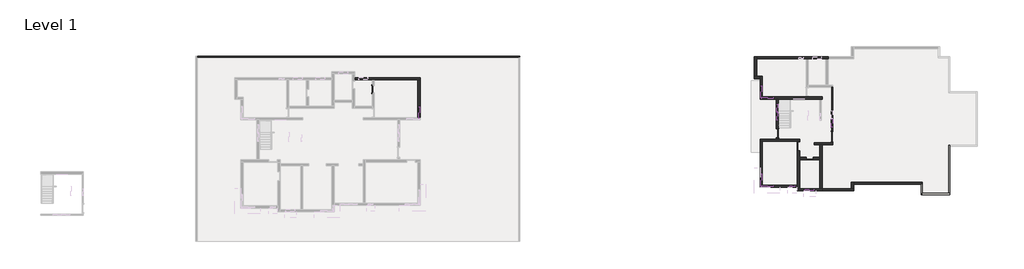
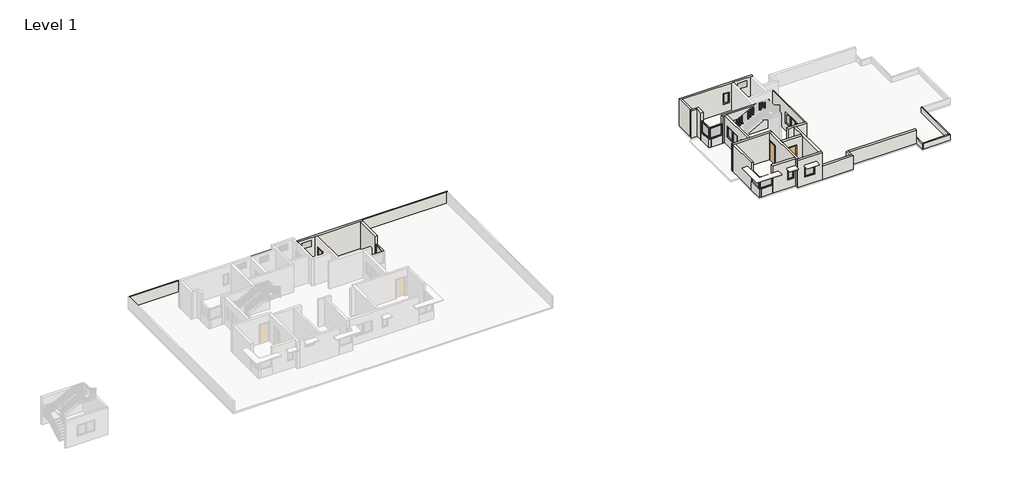
# One storey, part 3 of 9: 38 members, 29 walls, 12 plates, 5 doors.
"""IFC4 building model written with IfcOpenShell, lengths in millimetres."""

from ifc_helpers import new_model, si_unit, frame, origin, origin_with_axes, place, context, project, spatial, polyline, outline, extrude, faceted_brep, transform, mapped, element, save
from components import door_bb98abfd, single_flush_door_3_0ca8825f, door_e6ebe4aa, member_75074519, member_05917e3b, member_5783932f, member_49503176, member_cba00588, member_c17f1be2, member_2b49869a, member_8d24a278, member_86d06fe4, member_e557a406, system_panel_glazed_87944ff9, system_panel_glazed_c8a97ecb, system_panel_glazed_8ae75b46, system_panel_glazed_1b15d1ca, system_panel_glazed_cc4caca5, system_panel_glazed_25f99c47, system_panel_glazed_1bcf12e0, system_panel_glazed_610bb4e0

model = new_model("IFC4")

# Units and contexts
model_context = context("Model", 3, world=origin())
ifc_project = project(units=[si_unit("LENGTHUNIT", "METRE", prefix="MILLI")], contexts=[model_context])

# Site, building, storey
site = spatial("IfcSite", under=ifc_project)
building = spatial("IfcBuilding", under=site)
storey = spatial("IfcBuildingStorey", under=building, Name="Level 1", Elevation=0.0)

# Doors
placement = place(None, origin())
door_shape = door_bb98abfd(model_context)
element("IfcDoor", 1, ObjectType="Single-Flush : door 2'6\"", at=placement, inside=storey, context=model_context, shape_type="MappedRepresentation", body=[
    mapped(door_shape, transform((-29076.4146233, 18676.4624892, 0.0), x_axis=(0.0, 1.0, 0.0), y_axis=(-1.0, 0.0, 0.0), z_axis=(0.0, 0.0, 1.0))),
])
element("IfcDoor", 2, ObjectType="Single-Flush : door 2'6\"", at=placement, inside=storey, context=model_context, shape_type="MappedRepresentation", body=[
    mapped(door_shape, transform((16569.5100959, 11434.669664, 0.0), x_axis=(-1.0, 0.0, 0.0), y_axis=(0.0, -1.0, 0.0), z_axis=(0.0, 0.0, 1.0))),
])
single_flush_door_3_shape = single_flush_door_3_0ca8825f(model_context)
element("IfcDoor", 3, ObjectType="Single-Flush : door 3'", at=placement, inside=storey, context=model_context, shape_type="MappedRepresentation", body=[
    mapped(single_flush_door_3_shape, transform((13178.6100959, 14076.3480703, 0.0), x_axis=(0.0, -1.0, 0.0), y_axis=(1.0, 0.0, 0.0), z_axis=(0.0, 0.0, 1.0))),
])
element("IfcDoor", 4, ObjectType="Single-Flush : door 3'", at=placement, inside=storey, context=model_context, shape_type="MappedRepresentation", body=[
    mapped(single_flush_door_3_shape, transform((15388.4100959, 12704.7480703, 0.0), x_axis=(0.0, 1.0, 0.0), y_axis=(-1.0, 0.0, 0.0), z_axis=(0.0, 0.0, 1.0))),
])
door_2_shape = door_e6ebe4aa(model_context)
element("IfcDoor", 5, ObjectType="Single-Flush : door 3'6\"", at=placement, inside=storey, context=model_context, shape_type="MappedRepresentation", body=[
    mapped(door_2_shape, transform((18912.6600959, 13695.3480703, 0.0), x_axis=(0.0, -1.0, 0.0), y_axis=(1.0, 0.0, 0.0), z_axis=(0.0, 0.0, 1.0))),
])

# Members
member_shape = member_75074519(model_context)
element("IfcMember", 6, ObjectType="Rectangular Mullion : 2.5\" x 5\" rectangular", at=placement, inside=storey, context=model_context, shape_type="MappedRepresentation", body=[
    mapped(member_shape, transform((-24263.1146233, 16911.1624892, 914.4), x_axis=(0.0, 1.0, 0.0), y_axis=(1.0, 0.0, 0.0), z_axis=(0.0, 0.0, -1.0))),
])
element("IfcMember", 7, ObjectType="Rectangular Mullion : 2.5\" x 5\" rectangular", at=placement, inside=storey, context=model_context, shape_type="MappedRepresentation", body=[
    mapped(member_shape, transform((11486.0219681, 17689.4980703, 914.4), x_axis=(0.0, -1.0, 0.0), y_axis=(-1.0, 0.0, 0.0), z_axis=(0.0, 0.0, -1.0))),
])
element("IfcMember", 8, ObjectType="Rectangular Mullion : 2.5\" x 5\" rectangular", at=placement, inside=storey, context=model_context, shape_type="MappedRepresentation", body=[
    mapped(member_shape, transform((12835.7100959, 17752.9980703, 914.4), x_axis=(1.0, 0.0, 0.0), y_axis=(0.0, -1.0, 0.0), z_axis=(0.0, 0.0, -1.0))),
])
element("IfcMember", 9, ObjectType="Rectangular Mullion : 2.5\" x 5\" rectangular", at=placement, inside=storey, context=model_context, shape_type="MappedRepresentation", body=[
    mapped(member_shape, transform((11486.0219681, 8462.949831, 914.4), x_axis=(0.0, -1.0, 0.0), y_axis=(-1.0, 0.0, 0.0), z_axis=(0.0, 0.0, -1.0))),
])
element("IfcMember", 10, ObjectType="Rectangular Mullion : 2.5\" x 5\" rectangular", at=placement, inside=storey, context=model_context, shape_type="MappedRepresentation", body=[
    mapped(member_shape, transform((12835.7100959, 8526.449831, 914.4), x_axis=(1.0, 0.0, 0.0), y_axis=(0.0, -1.0, 0.0), z_axis=(0.0, 0.0, -1.0))),
])
element("IfcMember", 11, ObjectType="Rectangular Mullion : 2.5\" x 5\" rectangular", at=placement, inside=storey, context=model_context, shape_type="MappedRepresentation", body=[
    mapped(member_shape, transform((15045.5100959, 8513.7480703, 914.4), x_axis=(1.0, 0.0, 0.0), y_axis=(0.0, -1.0, 0.0), z_axis=(0.0, 0.0, -1.0))),
])
element("IfcMember", 12, ObjectType="Rectangular Mullion : 2.5\" x 5\" rectangular", at=placement, inside=storey, context=model_context, shape_type="MappedRepresentation", body=[
    mapped(member_shape, transform((17064.8100959, 8132.669664, 914.4), x_axis=(1.0, 0.0, 0.0), y_axis=(0.0, -1.0, 0.0), z_axis=(0.0, 0.0, -1.0))),
])
element("IfcMember", 13, ObjectType="Rectangular Mullion : 2.5\" x 5\" rectangular", at=placement, inside=storey, context=model_context, shape_type="MappedRepresentation", body=[
    mapped(member_shape, transform((11486.0219681, 19092.8480703, 2133.6), x_axis=(0.0, 1.0, 0.0), y_axis=(-1.0, 0.0, 0.0), z_axis=(0.0, 0.0, 1.0))),
])
element("IfcMember", 14, ObjectType="Rectangular Mullion : 2.5\" x 5\" rectangular", at=placement, inside=storey, context=model_context, shape_type="MappedRepresentation", body=[
    mapped(member_shape, transform((11486.0219681, 17752.9980703, 2133.6), x_axis=(-1.0, 0.0, 0.0), y_axis=(0.0, -1.0, 0.0), z_axis=(0.0, 0.0, 1.0))),
])
element("IfcMember", 15, ObjectType="Rectangular Mullion : 2.5\" x 5\" rectangular", at=placement, inside=storey, context=model_context, shape_type="MappedRepresentation", body=[
    mapped(member_shape, transform((11486.0219681, 9872.649831, 2133.6), x_axis=(0.0, 1.0, 0.0), y_axis=(-1.0, 0.0, 0.0), z_axis=(0.0, 0.0, 1.0))),
])
element("IfcMember", 16, ObjectType="Rectangular Mullion : 2.5\" x 5\" rectangular", at=placement, inside=storey, context=model_context, shape_type="MappedRepresentation", body=[
    mapped(member_shape, transform((11486.0219681, 8526.449831, 2133.6), x_axis=(-1.0, 0.0, 0.0), y_axis=(0.0, -1.0, 0.0), z_axis=(0.0, 0.0, 1.0))),
])
element("IfcMember", 17, ObjectType="Rectangular Mullion : 2.5\" x 5\" rectangular", at=placement, inside=storey, context=model_context, shape_type="MappedRepresentation", body=[
    mapped(member_shape, transform((14435.9100959, 8513.7480703, 2133.6), x_axis=(-1.0, 0.0, 0.0), y_axis=(0.0, -1.0, 0.0), z_axis=(0.0, 0.0, 1.0))),
])
element("IfcMember", 18, ObjectType="Rectangular Mullion : 2.5\" x 5\" rectangular", at=placement, inside=storey, context=model_context, shape_type="MappedRepresentation", body=[
    mapped(member_shape, transform((15998.0100959, 8132.669664, 2133.6), x_axis=(-1.0, 0.0, 0.0), y_axis=(0.0, -1.0, 0.0), z_axis=(0.0, 0.0, 1.0))),
])
member_2_shape = member_05917e3b(model_context)
element("IfcMember", 19, ObjectType="Rectangular Mullion : 2.5\" x 5\" rectangular", at=placement, inside=storey, context=model_context, shape_type="MappedRepresentation", body=[
    mapped(member_2_shape, transform((12772.2100959, 17752.9980703, 2133.6), x_axis=(0.0, 0.0, 1.0), y_axis=(0.0, -1.0, 0.0), z_axis=(1.0, 0.0, 0.0))),
])
element("IfcMember", 20, ObjectType="Rectangular Mullion : 2.5\" x 5\" rectangular", at=placement, inside=storey, context=model_context, shape_type="MappedRepresentation", body=[
    mapped(member_2_shape, transform((12772.2100959, 8526.449831, 2133.6), x_axis=(0.0, 0.0, 1.0), y_axis=(0.0, -1.0, 0.0), z_axis=(1.0, 0.0, 0.0))),
])
element("IfcMember", 21, ObjectType="Rectangular Mullion : 2.5\" x 5\" rectangular", at=placement, inside=storey, context=model_context, shape_type="MappedRepresentation", body=[
    mapped(member_2_shape, transform((11549.5219681, 17752.9980703, 914.4), x_axis=(0.0, 0.0, -1.0), y_axis=(0.0, -1.0, 0.0), z_axis=(-1.0, 0.0, 0.0))),
])
element("IfcMember", 22, ObjectType="Rectangular Mullion : 2.5\" x 5\" rectangular", at=placement, inside=storey, context=model_context, shape_type="MappedRepresentation", body=[
    mapped(member_2_shape, transform((11549.5219681, 8526.449831, 914.4), x_axis=(0.0, 0.0, -1.0), y_axis=(0.0, -1.0, 0.0), z_axis=(-1.0, 0.0, 0.0))),
])
member_3_shape = member_5783932f(model_context)
element("IfcMember", 23, ObjectType="Rectangular Mullion : 2.5\" x 5\" rectangular", at=placement, inside=storey, context=model_context, shape_type="MappedRepresentation", body=[
    mapped(member_3_shape, transform((11486.0219681, 8526.449831, 2133.6), x_axis=(0.0, 0.0, 1.0), y_axis=(-1.0, 0.0, 0.0), z_axis=(0.0, -1.0, 0.0))),
])
element("IfcMember", 24, ObjectType="Rectangular Mullion : 2.5\" x 5\" rectangular", at=placement, inside=storey, context=model_context, shape_type="MappedRepresentation", body=[
    mapped(member_3_shape, transform((11486.0219681, 9809.149831, 914.4), x_axis=(0.0, 0.0, -1.0), y_axis=(-1.0, 0.0, 0.0), z_axis=(0.0, 1.0, 0.0))),
])
member_4_shape = member_49503176(model_context)
element("IfcMember", 25, ObjectType="Rectangular Mullion : 2.5\" x 5\" rectangular", at=placement, inside=storey, context=model_context, shape_type="MappedRepresentation", body=[
    mapped(member_4_shape, transform((-24263.1146233, 16847.6624892, 2133.6), x_axis=(0.0, 0.0, 1.0), y_axis=(1.0, 0.0, 0.0), z_axis=(0.0, 1.0, 0.0))),
])
member_5_shape = member_cba00588(model_context)
element("IfcMember", 26, ObjectType="Rectangular Mullion : 2.5\" x 5\" rectangular", at=placement, inside=storey, context=model_context, shape_type="MappedRepresentation", body=[
    mapped(member_5_shape, transform((11486.0219681, 17752.9980703, 2133.6), x_axis=(0.0, 0.0, 1.0), y_axis=(-1.0, 0.0, 0.0), z_axis=(0.0, -1.0, 0.0))),
])
element("IfcMember", 27, ObjectType="Rectangular Mullion : 2.5\" x 5\" rectangular", at=placement, inside=storey, context=model_context, shape_type="MappedRepresentation", body=[
    mapped(member_5_shape, transform((11486.0219681, 19029.3480703, 914.4), x_axis=(0.0, 0.0, -1.0), y_axis=(-1.0, 0.0, 0.0), z_axis=(0.0, 1.0, 0.0))),
])
member_6_shape = member_c17f1be2(model_context)
element("IfcMember", 28, ObjectType="Rectangular Mullion : 2.5\" x 5\" rectangular", at=placement, inside=storey, context=model_context, shape_type="MappedRepresentation", body=[
    mapped(member_6_shape, transform((13162.4368388, 17124.3480703, 2133.6), x_axis=(0.0, 0.0, 1.0), y_axis=(1.0, 0.0, 0.0), z_axis=(0.0, 1.0, 0.0))),
])
element("IfcMember", 29, ObjectType="Rectangular Mullion : 2.5\" x 5\" rectangular", at=placement, inside=storey, context=model_context, shape_type="MappedRepresentation", body=[
    mapped(member_6_shape, transform((13162.4368388, 16241.6980703, 2133.6), x_axis=(0.0, 0.0, 1.0), y_axis=(1.0, 0.0, 0.0), z_axis=(0.0, 1.0, 0.0))),
])
element("IfcMember", 30, ObjectType="Rectangular Mullion : 2.5\" x 5\" rectangular", at=placement, inside=storey, context=model_context, shape_type="MappedRepresentation", body=[
    mapped(member_6_shape, transform((13162.4368388, 15422.5480703, 914.4), x_axis=(0.0, 0.0, -1.0), y_axis=(1.0, 0.0, 0.0), z_axis=(0.0, -1.0, 0.0))),
])
element("IfcMember", 31, ObjectType="Rectangular Mullion : 2.5\" x 5\" rectangular", at=placement, inside=storey, context=model_context, shape_type="MappedRepresentation", body=[
    mapped(member_6_shape, transform((13162.4368388, 16305.1980703, 914.4), x_axis=(0.0, 0.0, -1.0), y_axis=(1.0, 0.0, 0.0), z_axis=(0.0, -1.0, 0.0))),
])
member_7_shape = member_2b49869a(model_context)
element("IfcMember", 32, ObjectType="Rectangular Mullion : 2.5\" x 5\" rectangular", at=placement, inside=storey, context=model_context, shape_type="MappedRepresentation", body=[
    mapped(member_7_shape, transform((13162.4368388, 16273.4480703, 914.4), x_axis=(0.0, 1.0, 0.0), y_axis=(1.0, 0.0, 0.0), z_axis=(0.0, 0.0, -1.0))),
])
element("IfcMember", 33, ObjectType="Rectangular Mullion : 2.5\" x 5\" rectangular", at=placement, inside=storey, context=model_context, shape_type="MappedRepresentation", body=[
    mapped(member_7_shape, transform((18890.1839667, 15549.2510521, 914.4), x_axis=(0.0, 1.0, 0.0), y_axis=(1.0, 0.0, 0.0), z_axis=(0.0, 0.0, -1.0))),
])
element("IfcMember", 34, ObjectType="Rectangular Mullion : 2.5\" x 5\" rectangular", at=placement, inside=storey, context=model_context, shape_type="MappedRepresentation", body=[
    mapped(member_shape, transform((13162.4368388, 17187.8480703, 914.4), x_axis=(0.0, 1.0, 0.0), y_axis=(1.0, 0.0, 0.0), z_axis=(0.0, 0.0, -1.0))),
])
element("IfcMember", 35, ObjectType="Rectangular Mullion : 2.5\" x 5\" rectangular", at=placement, inside=storey, context=model_context, shape_type="MappedRepresentation", body=[
    mapped(member_shape, transform((13162.4368388, 15359.0480703, 2133.6), x_axis=(0.0, -1.0, 0.0), y_axis=(1.0, 0.0, 0.0), z_axis=(0.0, 0.0, 1.0))),
])
element("IfcMember", 36, ObjectType="Rectangular Mullion : 2.5\" x 5\" rectangular", at=placement, inside=storey, context=model_context, shape_type="MappedRepresentation", body=[
    mapped(member_shape, transform((18890.1839667, 14635.1480703, 2133.6), x_axis=(0.0, -1.0, 0.0), y_axis=(1.0, 0.0, 0.0), z_axis=(0.0, 0.0, 1.0))),
])
member_8_shape = member_8d24a278(model_context)
element("IfcMember", 37, ObjectType="Rectangular Mullion : 2.5\" x 5\" rectangular", at=placement, inside=storey, context=model_context, shape_type="MappedRepresentation", body=[
    mapped(member_8_shape, transform((18890.1839667, 15517.5010521, 2133.6), x_axis=(0.0, 0.0, 1.0), y_axis=(1.0, 0.0, 0.0), z_axis=(0.0, 1.0, 0.0))),
])
element("IfcMember", 38, ObjectType="Rectangular Mullion : 2.5\" x 5\" rectangular", at=placement, inside=storey, context=model_context, shape_type="MappedRepresentation", body=[
    mapped(member_8_shape, transform((18890.1839667, 14698.6480703, 914.4), x_axis=(0.0, 0.0, -1.0), y_axis=(1.0, 0.0, 0.0), z_axis=(0.0, -1.0, 0.0))),
])
element("IfcMember", 39, ObjectType="Rectangular Mullion : 2.5\" x 5\" rectangular", at=placement, inside=storey, context=model_context, shape_type="MappedRepresentation", body=[
    mapped(member_8_shape, transform((18890.1839667, 15581.0010521, 914.4), x_axis=(0.0, 0.0, -1.0), y_axis=(1.0, 0.0, 0.0), z_axis=(0.0, -1.0, 0.0))),
])
member_9_shape = member_86d06fe4(model_context)
element("IfcMember", 40, ObjectType="Rectangular Mullion : 2.5\" x 5\" rectangular", at=placement, inside=storey, context=model_context, shape_type="MappedRepresentation", body=[
    mapped(member_9_shape, transform((14982.0100959, 8513.7480703, 2133.6), x_axis=(0.0, 0.0, 1.0), y_axis=(0.0, -1.0, 0.0), z_axis=(1.0, 0.0, 0.0))),
])
element("IfcMember", 41, ObjectType="Rectangular Mullion : 2.5\" x 5\" rectangular", at=placement, inside=storey, context=model_context, shape_type="MappedRepresentation", body=[
    mapped(member_9_shape, transform((14499.4100959, 8513.7480703, 914.4), x_axis=(0.0, 0.0, -1.0), y_axis=(0.0, -1.0, 0.0), z_axis=(-1.0, 0.0, 0.0))),
])
member_10_shape = member_e557a406(model_context)
element("IfcMember", 42, ObjectType="Rectangular Mullion : 2.5\" x 5\" rectangular", at=placement, inside=storey, context=model_context, shape_type="MappedRepresentation", body=[
    mapped(member_10_shape, transform((17001.3100959, 8132.669664, 2133.6), x_axis=(0.0, 0.0, 1.0), y_axis=(0.0, -1.0, 0.0), z_axis=(1.0, 0.0, 0.0))),
])
element("IfcMember", 43, ObjectType="Rectangular Mullion : 2.5\" x 5\" rectangular", at=placement, inside=storey, context=model_context, shape_type="MappedRepresentation", body=[
    mapped(member_10_shape, transform((16061.5100959, 8132.669664, 914.4), x_axis=(0.0, 0.0, -1.0), y_axis=(0.0, -1.0, 0.0), z_axis=(-1.0, 0.0, 0.0))),
])

# Plates
system_panel_glazed_shape = system_panel_glazed_87944ff9(model_context)
element("IfcPlate", 44, ObjectType="System Panel : Glazed", at=placement, inside=storey, context=model_context, shape_type="MappedRepresentation", body=[
    mapped(system_panel_glazed_shape, transform((11486.0219681, 9167.799831, 977.9), x_axis=(0.0, -1.0, 0.0), y_axis=(1.0, 0.0, 0.0), z_axis=(0.0, 0.0, 1.0))),
])
system_panel_glazed_2_shape = system_panel_glazed_c8a97ecb(model_context)
element("IfcPlate", 45, ObjectType="System Panel : Glazed", at=placement, inside=storey, context=model_context, shape_type="MappedRepresentation", body=[
    mapped(system_panel_glazed_2_shape, transform((12160.866032, 17752.9980703, 977.9), x_axis=(1.0, 0.0, 0.0), y_axis=(0.0, 1.0, 0.0), z_axis=(0.0, 0.0, 1.0))),
])
element("IfcPlate", 46, ObjectType="System Panel : Glazed", at=placement, inside=storey, context=model_context, shape_type="MappedRepresentation", body=[
    mapped(system_panel_glazed_2_shape, transform((12160.866032, 8526.449831, 977.9), x_axis=(1.0, 0.0, 0.0), y_axis=(0.0, 1.0, 0.0), z_axis=(0.0, 0.0, 1.0))),
])
system_panel_glazed_3_shape = system_panel_glazed_8ae75b46(model_context)
element("IfcPlate", 47, ObjectType="System Panel : Glazed", at=placement, inside=storey, context=model_context, shape_type="MappedRepresentation", body=[
    mapped(system_panel_glazed_3_shape, transform((-24263.1146233, 16231.7124892, 977.9), x_axis=(0.0, 1.0, 0.0), y_axis=(-1.0, 0.0, 0.0), z_axis=(0.0, 0.0, 1.0))),
])
system_panel_glazed_4_shape = system_panel_glazed_1b15d1ca(model_context)
element("IfcPlate", 48, ObjectType="System Panel : Glazed", at=placement, inside=storey, context=model_context, shape_type="MappedRepresentation", body=[
    mapped(system_panel_glazed_4_shape, transform((11486.0219681, 18391.1730703, 977.9), x_axis=(0.0, -1.0, 0.0), y_axis=(1.0, 0.0, 0.0), z_axis=(0.0, 0.0, 1.0))),
])
system_panel_glazed_5_shape = system_panel_glazed_cc4caca5(model_context)
element("IfcPlate", 49, ObjectType="System Panel : Glazed", at=placement, inside=storey, context=model_context, shape_type="MappedRepresentation", body=[
    mapped(system_panel_glazed_5_shape, transform((13162.4368388, 15832.1230703, 977.9), x_axis=(0.0, 1.0, 0.0), y_axis=(-1.0, 0.0, 0.0), z_axis=(0.0, 0.0, 1.0))),
])
element("IfcPlate", 50, ObjectType="System Panel : Glazed", at=placement, inside=storey, context=model_context, shape_type="MappedRepresentation", body=[
    mapped(system_panel_glazed_5_shape, transform((13162.4368388, 16714.7730703, 977.9), x_axis=(0.0, 1.0, 0.0), y_axis=(-1.0, 0.0, 0.0), z_axis=(0.0, 0.0, 1.0))),
])
system_panel_glazed_6_shape = system_panel_glazed_25f99c47(model_context)
element("IfcPlate", 51, ObjectType="System Panel : Glazed", at=placement, inside=storey, context=model_context, shape_type="MappedRepresentation", body=[
    mapped(system_panel_glazed_6_shape, transform((18890.1839667, 15108.0745612, 977.9), x_axis=(0.0, 1.0, 0.0), y_axis=(-1.0, 0.0, 0.0), z_axis=(0.0, 0.0, 1.0))),
])
element("IfcPlate", 52, ObjectType="System Panel : Glazed", at=placement, inside=storey, context=model_context, shape_type="MappedRepresentation", body=[
    mapped(system_panel_glazed_6_shape, transform((18890.1839667, 15990.4275429, 977.9), x_axis=(0.0, 1.0, 0.0), y_axis=(-1.0, 0.0, 0.0), z_axis=(0.0, 0.0, 1.0))),
])
system_panel_glazed_7_shape = system_panel_glazed_1bcf12e0(model_context)
element("IfcPlate", 53, ObjectType="System Panel : Glazed", at=placement, inside=storey, context=model_context, shape_type="MappedRepresentation", body=[
    mapped(system_panel_glazed_7_shape, transform((15655.1100959, 21924.9480703, 977.9), x_axis=(1.0, 0.0, 0.0), y_axis=(0.0, 1.0, 0.0), z_axis=(0.0, 0.0, 1.0))),
])
element("IfcPlate", 54, ObjectType="System Panel : Glazed", at=placement, inside=storey, context=model_context, shape_type="MappedRepresentation", body=[
    mapped(system_panel_glazed_7_shape, transform((14740.7100959, 8513.7480703, 977.9), x_axis=(1.0, 0.0, 0.0), y_axis=(0.0, 1.0, 0.0), z_axis=(0.0, 0.0, 1.0))),
])
system_panel_glazed_8_shape = system_panel_glazed_610bb4e0(model_context)
element("IfcPlate", 55, ObjectType="System Panel : Glazed", at=placement, inside=storey, context=model_context, shape_type="MappedRepresentation", body=[
    mapped(system_panel_glazed_8_shape, transform((16531.4100959, 8132.669664, 977.9), x_axis=(1.0, 0.0, 0.0), y_axis=(0.0, 1.0, 0.0), z_axis=(0.0, 0.0, 1.0))),
])

# Walls
element("IfcWall", 56, at=placement, inside=storey, context=model_context, shape_type="Brep", body=[
    faceted_brep([(17864.9100959, 8043.769664, 0.0), (21141.5100959, 8043.769664, 0.0), (21141.5100959, 8043.769664, 1524.0), (17864.9100959, 8043.769664, 1524.0), (17864.9100959, 8272.369664, 0.0), (17864.9100959, 8272.369664, 1524.0), (20912.9100959, 8272.369664, 1524.0), (21141.5100959, 8272.369664, 1524.0), (21141.5100959, 8272.369664, 0.0), (20912.9100959, 8272.369664, 0.0)], [[[0, 1, 2, 3]], [[4, 5, 6, 7, 8, 9]], [[1, 0, 4, 9, 8]], [[3, 2, 7, 6, 5]], [[0, 3, 5, 4]], [[2, 1, 8, 7]]]),
])
element("IfcWall", 57, at=placement, inside=storey, context=model_context, shape_type="Brep", body=[
    faceted_brep([(21141.5100959, 8272.369664, 0.0), (21141.5100959, 8729.6480703, 0.0), (21141.5100959, 8958.2480703, 0.0), (21141.5100959, 8958.2480703, 1524.0), (21141.5100959, 8729.6480703, 1524.0), (21141.5100959, 8272.369664, 1524.0), (20912.9100959, 8272.369664, 0.0), (20912.9100959, 8272.369664, 1524.0), (20912.9100959, 8958.2480703, 1524.0), (20912.9100959, 8958.2480703, 0.0)], [[[0, 1, 2, 3, 4, 5]], [[6, 7, 8, 9]], [[2, 1, 0, 6, 9]], [[5, 4, 3, 8, 7]], [[0, 5, 7, 6]], [[3, 2, 9, 8]]]),
])
element("IfcWall", 58, at=placement, inside=storey, context=model_context, shape_type="Brep", body=[
    faceted_brep([(21141.5100959, 8729.6480703, 0.0), (28228.1100959, 8729.6480703, 0.0), (28228.1100959, 8729.6480703, 1524.0), (21141.5100959, 8729.6480703, 1524.0), (21141.5100959, 8958.2480703, 0.0), (21141.5100959, 8958.2480703, 1524.0), (28228.1100959, 8958.2480703, 1524.0), (28228.1100959, 8958.2480703, 609.6), (28228.1100959, 8958.2480703, 0.0)], [[[0, 1, 2, 3]], [[4, 5, 6, 7, 8]], [[1, 0, 4, 8]], [[3, 2, 6, 5]], [[0, 3, 5, 4]], [[2, 1, 8, 7, 6]]]),
])
element("IfcWall", 59, at=placement, inside=storey, context=model_context, shape_type="Brep", body=[
    faceted_brep([(28228.1100959, 8958.2480703, 0.0), (28228.1100959, 8729.6480703, 0.0), (28228.1100959, 7662.8480703, 0.0), (28228.1100959, 7662.8480703, 609.6), (28228.1100959, 8958.2480703, 609.6), (28342.4100959, 8958.2480703, 0.0), (28342.4100959, 8958.2480703, 609.6), (28342.4100959, 7777.1480703, 609.6), (28342.4100959, 7662.8480703, 609.6), (28342.4100959, 7662.8480703, 0.0), (28342.4100959, 7777.1480703, 0.0)], [[[0, 1, 2, 3, 4]], [[5, 6, 7, 8, 9, 10]], [[2, 1, 0, 5, 10, 9]], [[4, 3, 8, 7, 6]], [[0, 4, 6, 5]], [[3, 2, 9, 8]]]),
])
element("IfcWall", 60, at=placement, inside=storey, context=model_context, shape_type="Brep", body=[
    faceted_brep([(28342.4100959, 7662.8480703, 0.0), (31199.9100959, 7662.8480703, 0.0), (31199.9100959, 7662.8480703, 609.6), (28342.4100959, 7662.8480703, 609.6), (28342.4100959, 7777.1480703, 0.0), (28342.4100959, 7777.1480703, 609.6), (31085.6100959, 7777.1480703, 609.6), (31199.9100959, 7777.1480703, 609.6), (31199.9100959, 7777.1480703, 0.0), (31085.6100959, 7777.1480703, 0.0)], [[[0, 1, 2, 3]], [[4, 5, 6, 7, 8, 9]], [[1, 0, 4, 9, 8]], [[3, 2, 7, 6, 5]], [[0, 3, 5, 4]], [[2, 1, 8, 7]]]),
])
element("IfcWall", 61, at=placement, inside=storey, context=model_context, shape_type="Brep", body=[
    faceted_brep([(31199.9100959, 7777.1480703, 0.0), (31199.9100959, 12692.0480703, 0.0), (31199.9100959, 12806.3480703, 0.0), (31199.9100959, 12806.3480703, 609.6), (31199.9100959, 12692.0480703, 609.6), (31199.9100959, 7777.1480703, 609.6), (31085.6100959, 7777.1480703, 0.0), (31085.6100959, 7777.1480703, 609.6), (31085.6100959, 12806.3480703, 609.6), (31085.6100959, 12806.3480703, 0.0)], [[[0, 1, 2, 3, 4, 5]], [[6, 7, 8, 9]], [[2, 1, 0, 6, 9]], [[5, 4, 3, 8, 7]], [[0, 5, 7, 6]], [[3, 2, 9, 8]]]),
])
element("IfcWall", 62, at=placement, inside=storey, context=model_context, shape_type="Brep", body=[
    faceted_brep([(-47478.7146233, 22016.5624892, 0.0), (-13874.5146233, 22016.5624892, 0.0), (-13760.2146233, 22016.5624892, 0.0), (-13760.2146233, 22016.5624892, 1219.2), (-13874.5146233, 22016.5624892, 1219.2), (-47478.7146233, 22016.5624892, 1219.2), (-47478.7146233, 22130.8624892, 0.0), (-47478.7146233, 22130.8624892, 1219.2), (-13760.2146233, 22130.8624892, 1219.2), (-13760.2146233, 22130.8624892, 0.0)], [[[0, 1, 2, 3, 4, 5]], [[6, 7, 8, 9]], [[2, 1, 0, 6, 9]], [[5, 4, 3, 8, 7]], [[0, 5, 7, 6]], [[3, 2, 9, 8]]]),
])
element("IfcWall", 63, ObjectType="WALL 9\"", at=placement, inside=storey, context=model_context, shape_type="Brep", body=[
    faceted_brep([(-31019.5146233, 19654.3624892, 0.0), (-29190.7146233, 19654.3624892, 0.0), (-28962.1146233, 19654.3624892, 0.0), (-24390.1146233, 19654.3624892, 0.0), (-24161.5146233, 19654.3624892, 0.0), (-24161.5146233, 19654.3624892, 3048.0), (-24390.1146233, 19654.3624892, 3048.0), (-28962.1146233, 19654.3624892, 3048.0), (-29190.7146233, 19654.3624892, 3048.0), (-31019.5146233, 19654.3624892, 3048.0), (-30562.3146233, 19654.3624892, 2743.2), (-29647.9146233, 19654.3624892, 2743.2), (-29647.9146233, 19654.3624892, 2133.6), (-30562.3146233, 19654.3624892, 2133.6), (-31019.5146233, 19882.9624892, 0.0), (-31019.5146233, 19882.9624892, 3048.0), (-24161.5146233, 19882.9624892, 3048.0), (-24161.5146233, 19882.9624892, 0.0), (-30562.3146233, 19882.9624892, 2743.2), (-30562.3146233, 19882.9624892, 2133.6), (-29647.9146233, 19882.9624892, 2133.6), (-29647.9146233, 19882.9624892, 2743.2)], [[[0, 1, 2, 3, 4, 5, 6, 7, 8, 9], [10, 11, 12, 13]], [[14, 15, 16, 17], [18, 19, 20, 21]], [[4, 3, 2, 1, 0, 14, 17]], [[9, 8, 7, 6, 5, 16, 15]], [[0, 9, 15, 14]], [[5, 4, 17, 16]], [[19, 18, 10, 13]], [[20, 19, 13, 12]], [[21, 20, 12, 11]], [[18, 21, 11, 10]]]),
])
element("IfcWall", 64, ObjectType="WALL 9\"", at=placement, inside=storey, context=model_context, shape_type="Brep", body=[
    faceted_brep([(11616.5100959, 19092.8480703, 3048.0), (11616.5100959, 19092.8480703, 2133.6), (11616.5100959, 19092.8480703, 914.4), (11616.5100959, 19092.8480703, 0.0), (11616.5100959, 20007.2480703, 0.0), (11616.5100959, 20007.2480703, 3048.0), (11387.9100959, 19092.8480703, 0.0), (11387.9100959, 19092.8480703, 914.4), (11387.9100959, 19092.8480703, 2133.6), (11387.9100959, 19092.8480703, 3048.0), (11387.9100959, 19778.6480703, 3048.0), (11387.9100959, 20007.2480703, 3048.0), (11387.9100959, 20007.2480703, 0.0), (11387.9100959, 19778.6480703, 0.0)], [[[0, 1, 2, 3, 4, 5]], [[6, 7, 8, 9, 10, 11, 12, 13]], [[4, 3, 6, 13, 12]], [[5, 4, 12, 11]], [[0, 9, 8, 7, 6, 3, 2, 1]], [[0, 5, 11, 10, 9]]]),
])
element("IfcWall", 65, ObjectType="WALL 9\"", at=placement, inside=storey, context=model_context, shape_type="Brep", body=[
    faceted_brep([(11387.9100959, 20007.2480703, 0.0), (11006.9100959, 20007.2480703, 0.0), (10778.3100959, 20007.2480703, 0.0), (10778.3100959, 20007.2480703, 3048.0), (11006.9100959, 20007.2480703, 3048.0), (11387.9100959, 20007.2480703, 3048.0), (11387.9100959, 19778.6480703, 0.0), (11387.9100959, 19778.6480703, 3048.0), (10778.3100959, 19778.6480703, 3048.0), (10778.3100959, 19778.6480703, 0.0)], [[[0, 1, 2, 3, 4, 5]], [[6, 7, 8, 9]], [[2, 1, 0, 6, 9]], [[0, 5, 7, 6]], [[3, 2, 9, 8]], [[5, 4, 3, 8, 7]]]),
])
element("IfcWall", 66, ObjectType="WALL 9\"", at=placement, inside=storey, context=model_context, shape_type="Brep", body=[
    faceted_brep([(11006.9100959, 20007.2480703, 0.0), (11006.9100959, 21836.0480703, 0.0), (11006.9100959, 22064.6480703, 0.0), (11006.9100959, 22064.6480703, 3048.0), (11006.9100959, 21836.0480703, 3048.0), (11006.9100959, 20007.2480703, 3048.0), (10778.3100959, 20007.2480703, 0.0), (10778.3100959, 20007.2480703, 3048.0), (10778.3100959, 22064.6480703, 3048.0), (10778.3100959, 22064.6480703, 0.0)], [[[0, 1, 2, 3, 4, 5]], [[6, 7, 8, 9]], [[2, 1, 0, 6, 9]], [[0, 5, 7, 6]], [[3, 2, 9, 8]], [[5, 4, 3, 8, 7]]]),
])
element("IfcWall", 67, ObjectType="WALL 9\"", at=placement, inside=storey, context=model_context, shape_type="Brep", body=[
    faceted_brep([(11006.9100959, 21836.0480703, 0.0), (16188.5100959, 21836.0480703, 0.0), (16417.1100959, 21836.0480703, 0.0), (18245.9100959, 21836.0480703, 0.0), (18474.5100959, 21836.0480703, 0.0), (18474.5100959, 21836.0480703, 1524.0), (18474.5100959, 21836.0480703, 3048.0), (18245.9100959, 21836.0480703, 3048.0), (16417.1100959, 21836.0480703, 3048.0), (16188.5100959, 21836.0480703, 3048.0), (11006.9100959, 21836.0480703, 3048.0), (15350.3100959, 21836.0480703, 914.4), (15350.3100959, 21836.0480703, 2133.6), (15959.9100959, 21836.0480703, 2133.6), (15959.9100959, 21836.0480703, 914.4), (16874.3100959, 21836.0480703, 2133.6), (16874.3100959, 21836.0480703, 2743.2), (17788.7100959, 21836.0480703, 2743.2), (17788.7100959, 21836.0480703, 2133.6), (18474.5100959, 22064.6480703, 0.0), (11006.9100959, 22064.6480703, 0.0), (11006.9100959, 22064.6480703, 3048.0), (18474.5100959, 22064.6480703, 3048.0), (18474.5100959, 22064.6480703, 1524.0), (15350.3100959, 22064.6480703, 2133.6), (15350.3100959, 22064.6480703, 914.4), (15959.9100959, 22064.6480703, 914.4), (15959.9100959, 22064.6480703, 2133.6), (16874.3100959, 22064.6480703, 2743.2), (16874.3100959, 22064.6480703, 2133.6), (17788.7100959, 22064.6480703, 2133.6), (17788.7100959, 22064.6480703, 2743.2)], [[[0, 1, 2, 3, 4, 5, 6, 7, 8, 9, 10], [11, 12, 13, 14], [15, 16, 17, 18]], [[19, 20, 21, 22, 23], [24, 25, 26, 27], [28, 29, 30, 31]], [[4, 3, 2, 1, 0, 20, 19]], [[0, 10, 21, 20]], [[4, 19, 23, 22, 6, 5]], [[11, 25, 24, 12]], [[12, 24, 27, 13]], [[13, 27, 26, 14]], [[25, 11, 14, 26]], [[29, 28, 16, 15]], [[30, 29, 15, 18]], [[31, 30, 18, 17]], [[28, 31, 17, 16]], [[10, 9, 8, 7, 6, 22, 21]]]),
])
element("IfcWall", 68, ObjectType="WALL 9\"", at=placement, inside=storey, context=model_context, shape_type="Brep", body=[
    faceted_brep([(12835.7100959, 17645.0480703, 3048.0), (12835.7100959, 17645.0480703, 2133.6), (12835.7100959, 17645.0480703, 914.4), (12835.7100959, 17645.0480703, 0.0), (13064.3100959, 17645.0480703, 0.0), (13292.9100959, 17645.0480703, 0.0), (17636.3100959, 17645.0480703, 0.0), (17750.6100959, 17645.0480703, 0.0), (17864.9100959, 17645.0480703, 0.0), (17864.9100959, 17645.0480703, 3048.0), (17750.6100959, 17645.0480703, 3048.0), (17636.3100959, 17645.0480703, 3048.0), (13292.9100959, 17645.0480703, 3048.0), (13064.3100959, 17645.0480703, 3048.0), (12835.7100959, 17873.6480703, 0.0), (12835.7100959, 17873.6480703, 914.4), (12835.7100959, 17873.6480703, 2133.6), (12835.7100959, 17873.6480703, 3048.0), (16188.5100959, 17873.6480703, 3048.0), (16417.1100959, 17873.6480703, 3048.0), (17864.9100959, 17873.6480703, 3048.0), (17864.9100959, 17873.6480703, 0.0), (16417.1100959, 17873.6480703, 0.0), (16188.5100959, 17873.6480703, 0.0)], [[[0, 1, 2, 3, 4, 5, 6, 7, 8, 9, 10, 11, 12, 13]], [[14, 15, 16, 17, 18, 19, 20, 21, 22, 23]], [[8, 7, 6, 5, 4, 3, 14, 23, 22, 21]], [[9, 8, 21, 20]], [[0, 17, 16, 15, 14, 3, 2, 1]], [[0, 13, 12, 11, 10, 9, 20, 19, 18, 17]]]),
])
element("IfcWall", 69, ObjectType="WALL 9\"", at=placement, inside=storey, context=model_context, shape_type="Brep", body=[
    faceted_brep([(13064.3100959, 17645.0480703, 3048.0), (13064.3100959, 17645.0480703, 0.0), (13064.3100959, 14533.5480703, 0.0), (13064.3100959, 14533.5480703, 2133.6), (13064.3100959, 13619.1480703, 2133.6), (13064.3100959, 13619.1480703, 0.0), (13064.3100959, 13454.0480703, 0.0), (13064.3100959, 13454.0480703, 3048.0), (13064.3100959, 15359.0480703, 2133.6), (13064.3100959, 15359.0480703, 914.4), (13064.3100959, 17187.8480703, 914.4), (13064.3100959, 17187.8480703, 2133.6), (13292.9100959, 17645.0480703, 0.0), (13292.9100959, 17645.0480703, 3048.0), (13292.9100959, 14647.8480703, 3048.0), (13292.9100959, 13454.0480703, 3048.0), (13292.9100959, 13454.0480703, 0.0), (13292.9100959, 13619.1480703, 0.0), (13292.9100959, 13619.1480703, 2133.6), (13292.9100959, 14533.5480703, 2133.6), (13292.9100959, 14533.5480703, 0.0), (13292.9100959, 15359.0480703, 914.4), (13292.9100959, 15359.0480703, 2133.6), (13292.9100959, 17187.8480703, 2133.6), (13292.9100959, 17187.8480703, 914.4)], [[[0, 1, 2, 3, 4, 5, 6, 7], [8, 9, 10, 11]], [[12, 13, 14, 15, 16, 17, 18, 19, 20], [21, 22, 23, 24]], [[1, 12, 20, 2]], [[16, 6, 5, 17]], [[1, 0, 13, 12]], [[7, 6, 16, 15]], [[21, 9, 8, 22]], [[22, 8, 11, 23]], [[23, 11, 10, 24]], [[9, 21, 24, 10]], [[18, 17, 5, 4]], [[19, 18, 4, 3]], [[20, 19, 3, 2]], [[13, 0, 7, 15, 14]]]),
])
element("IfcWall", 70, ObjectType="WALL 9\"", at=placement, inside=storey, context=model_context, shape_type="Brep", body=[
    faceted_brep([(11387.9100959, 13225.4480703, 0.0), (11616.5100959, 13225.4480703, 0.0), (15274.1100959, 13225.4480703, 0.0), (15502.7100959, 13225.4480703, 0.0), (15502.7100959, 13225.4480703, 3048.0), (15274.1100959, 13225.4480703, 3048.0), (11616.5100959, 13225.4480703, 3048.0), (11387.9100959, 13225.4480703, 3048.0), (11387.9100959, 13454.0480703, 0.0), (11387.9100959, 13454.0480703, 3048.0), (13064.3100959, 13454.0480703, 3048.0), (13292.9100959, 13454.0480703, 3048.0), (15502.7100959, 13454.0480703, 3048.0), (15502.7100959, 13454.0480703, 0.0), (13292.9100959, 13454.0480703, 0.0), (13064.3100959, 13454.0480703, 0.0)], [[[0, 1, 2, 3, 4, 5, 6, 7]], [[8, 9, 10, 11, 12, 13, 14, 15]], [[3, 2, 1, 0, 8, 15, 14, 13]], [[0, 7, 9, 8]], [[4, 3, 13, 12]], [[7, 6, 5, 4, 12, 11, 10, 9]]]),
])
element("IfcWall", 71, ObjectType="WALL 9\"", at=placement, inside=storey, context=model_context, shape_type="Brep", body=[
    faceted_brep([(11387.9100959, 13225.4480703, 0.0), (11387.9100959, 9872.649831, 0.0), (11387.9100959, 9872.649831, 914.4), (11387.9100959, 9872.649831, 2133.6), (11387.9100959, 9872.649831, 3048.0), (11387.9100959, 13225.4480703, 3048.0), (11616.5100959, 13225.4480703, 0.0), (11616.5100959, 13225.4480703, 3048.0), (11616.5100959, 9872.649831, 3048.0), (11616.5100959, 9872.649831, 2133.6), (11616.5100959, 9872.649831, 914.4), (11616.5100959, 9872.649831, 0.0)], [[[0, 1, 2, 3, 4, 5]], [[6, 7, 8, 9, 10, 11]], [[1, 0, 6, 11]], [[0, 5, 7, 6]], [[1, 11, 10, 9, 8, 4, 3, 2]], [[5, 4, 8, 7]]]),
])
element("IfcWall", 72, ObjectType="WALL 9\"", at=placement, inside=storey, context=model_context, shape_type="Brep", body=[
    faceted_brep([(12835.7100959, 8424.8480703, 0.0), (15274.1100959, 8424.8480703, 0.0), (15274.1100959, 8424.8480703, 3048.0), (12835.7100959, 8424.8480703, 3048.0), (12835.7100959, 8424.8480703, 2133.6), (12835.7100959, 8424.8480703, 914.4), (14435.9100959, 8424.8480703, 914.4), (14435.9100959, 8424.8480703, 2133.6), (15045.5100959, 8424.8480703, 2133.6), (15045.5100959, 8424.8480703, 914.4), (15274.1100959, 8653.4480703, 0.0), (12835.7100959, 8653.4480703, 0.0), (12835.7100959, 8653.4480703, 914.4), (12835.7100959, 8653.4480703, 2133.6), (12835.7100959, 8653.4480703, 3048.0), (15274.1100959, 8653.4480703, 3048.0), (14435.9100959, 8653.4480703, 2133.6), (14435.9100959, 8653.4480703, 914.4), (15045.5100959, 8653.4480703, 914.4), (15045.5100959, 8653.4480703, 2133.6)], [[[0, 1, 2, 3, 4, 5], [6, 7, 8, 9]], [[10, 11, 12, 13, 14, 15], [16, 17, 18, 19]], [[1, 0, 11, 10]], [[2, 1, 10, 15]], [[11, 0, 5, 4, 3, 14, 13, 12]], [[6, 17, 16, 7]], [[7, 16, 19, 8]], [[8, 19, 18, 9]], [[17, 6, 9, 18]], [[3, 2, 15, 14]]]),
])
element("IfcWall", 73, ObjectType="WALL 9\"", at=placement, inside=storey, context=model_context, shape_type="Brep", body=[
    faceted_brep([(15274.1100959, 8043.769664, 0.0), (17864.9100959, 8043.769664, 0.0), (17864.9100959, 8043.769664, 1524.0), (17864.9100959, 8043.769664, 3048.0), (15274.1100959, 8043.769664, 3048.0), (15998.0100959, 8043.769664, 914.4), (15998.0100959, 8043.769664, 2133.6), (17064.8100959, 8043.769664, 2133.6), (17064.8100959, 8043.769664, 914.4), (17864.9100959, 8272.369664, 0.0), (17636.3100959, 8272.369664, 0.0), (15502.7100959, 8272.369664, 0.0), (15274.1100959, 8272.369664, 0.0), (15274.1100959, 8272.369664, 3048.0), (15502.7100959, 8272.369664, 3048.0), (17636.3100959, 8272.369664, 3048.0), (17864.9100959, 8272.369664, 3048.0), (17864.9100959, 8272.369664, 1524.0), (15998.0100959, 8272.369664, 2133.6), (15998.0100959, 8272.369664, 914.4), (17064.8100959, 8272.369664, 914.4), (17064.8100959, 8272.369664, 2133.6)], [[[0, 1, 2, 3, 4], [5, 6, 7, 8]], [[9, 10, 11, 12, 13, 14, 15, 16, 17], [18, 19, 20, 21]], [[1, 0, 12, 11, 10, 9]], [[0, 4, 13, 12]], [[1, 9, 17, 16, 3, 2]], [[5, 19, 18, 6]], [[6, 18, 21, 7]], [[7, 21, 20, 8]], [[19, 5, 8, 20]], [[4, 3, 16, 15, 14, 13]]]),
])
element("IfcWall", 74, ObjectType="WALL 9\"", at=placement, inside=storey, context=model_context, shape_type="Brep", body=[
    faceted_brep([(17864.9100959, 8272.369664, 3048.0), (17864.9100959, 8272.369664, 0.0), (17864.9100959, 12844.4480703, 0.0), (17864.9100959, 12844.4480703, 3048.0), (17636.3100959, 8272.369664, 0.0), (17636.3100959, 8272.369664, 3048.0), (17636.3100959, 11320.369664, 3048.0), (17636.3100959, 11548.969664, 3048.0), (17636.3100959, 12844.4480703, 3048.0), (17636.3100959, 12844.4480703, 0.0), (17636.3100959, 11548.969664, 0.0), (17636.3100959, 11320.369664, 0.0)], [[[0, 1, 2, 3]], [[4, 5, 6, 7, 8, 9, 10, 11]], [[2, 1, 4, 11, 10, 9]], [[3, 2, 9, 8]], [[0, 5, 4, 1]], [[0, 3, 8, 7, 6, 5]]]),
])
element("IfcWall", 75, ObjectType="WALL 9\"", at=placement, inside=storey, context=model_context, shape_type="Brep", body=[
    faceted_brep([(15502.7100959, 13161.9480703, 2133.6), (15502.7100959, 13161.9480703, 0.0), (15502.7100959, 13225.4480703, 0.0), (15502.7100959, 13225.4480703, 3048.0), (15502.7100959, 11548.969664, 3048.0), (15502.7100959, 11320.369664, 3048.0), (15502.7100959, 8272.369664, 3048.0), (15502.7100959, 8272.369664, 0.0), (15502.7100959, 11320.369664, 0.0), (15502.7100959, 11548.969664, 0.0), (15502.7100959, 12247.5480703, 0.0), (15502.7100959, 12247.5480703, 2133.6), (15274.1100959, 13225.4480703, 0.0), (15274.1100959, 13161.9480703, 0.0), (15274.1100959, 13161.9480703, 2133.6), (15274.1100959, 12247.5480703, 2133.6), (15274.1100959, 12247.5480703, 0.0), (15274.1100959, 8653.4480703, 0.0), (15274.1100959, 8424.8480703, 0.0), (15274.1100959, 8272.369664, 0.0), (15274.1100959, 8272.369664, 3048.0), (15274.1100959, 8424.8480703, 3048.0), (15274.1100959, 8653.4480703, 3048.0), (15274.1100959, 13225.4480703, 3048.0)], [[[0, 1, 2, 3, 4, 5, 6, 7, 8, 9, 10, 11]], [[12, 13, 14, 15, 16, 17, 18, 19, 20, 21, 22, 23]], [[2, 1, 13, 12]], [[10, 9, 8, 7, 19, 18, 17, 16]], [[3, 2, 12, 23]], [[7, 6, 20, 19]], [[14, 13, 1, 0]], [[15, 14, 0, 11]], [[16, 15, 11, 10]], [[6, 5, 4, 3, 23, 22, 21, 20]]]),
])
element("IfcWall", 76, ObjectType="WALL 9\"", at=placement, inside=storey, context=model_context, shape_type="SweptSolid", body=[
    extrude(outline(polyline([(0.0, 15502.7100959), (0.0, 16188.5100959), (2133.6, 16188.5100959), (2133.6, 16950.5100959), (0.0, 16950.5100959), (0.0, 17636.3100959), (3048.0, 17636.3100959), (3048.0, 15502.7100959), (0.0, 15502.7100959)])), frame((0.0, 11320.369664, 0.0), z_axis=(0.0, 1.0, 0.0), x_axis=(0.0, 0.0, 1.0)), (0.0, 0.0, 1.0), 228.6),
])
element("IfcWall", 77, ObjectType="WALL 9\"", at=placement, inside=storey, context=model_context, shape_type="Brep", body=[
    faceted_brep([(17026.7100959, 12844.4480703, 0.0), (17636.3100959, 12844.4480703, 0.0), (17864.9100959, 12844.4480703, 0.0), (18969.8100959, 12844.4480703, 0.0), (18969.8100959, 12844.4480703, 3048.0), (17864.9100959, 12844.4480703, 3048.0), (17636.3100959, 12844.4480703, 3048.0), (17026.7100959, 12844.4480703, 3048.0), (17026.7100959, 13073.0480703, 0.0), (17026.7100959, 13073.0480703, 3048.0), (18855.5100959, 13073.0480703, 3048.0), (18969.8100959, 13073.0480703, 3048.0), (18969.8100959, 13073.0480703, 0.0), (18855.5100959, 13073.0480703, 0.0)], [[[0, 1, 2, 3, 4, 5, 6, 7]], [[8, 9, 10, 11, 12, 13]], [[3, 2, 1, 0, 8, 13, 12]], [[0, 7, 9, 8]], [[4, 3, 12, 11]], [[7, 6, 5, 4, 11, 10, 9]]]),
])
element("IfcWall", 78, ObjectType="WALL 9\" 2", at=placement, inside=storey, context=model_context, shape_type="Brep", body=[
    faceted_brep([(-24161.5146233, 16911.1624892, 3048.0), (-24161.5146233, 16911.1624892, 2133.6), (-24161.5146233, 16911.1624892, 914.4), (-24161.5146233, 16911.1624892, 0.0), (-24161.5146233, 19654.3624892, 0.0), (-24161.5146233, 19654.3624892, 3048.0), (-24390.1146233, 16911.1624892, 0.0), (-24390.1146233, 16911.1624892, 914.4), (-24390.1146233, 16911.1624892, 2133.6), (-24390.1146233, 16911.1624892, 3048.0), (-24390.1146233, 19654.3624892, 3048.0), (-24390.1146233, 19654.3624892, 0.0)], [[[0, 1, 2, 3, 4, 5]], [[6, 7, 8, 9, 10, 11]], [[4, 3, 6, 11]], [[0, 5, 10, 9]], [[5, 4, 11, 10]], [[0, 9, 8, 7, 6, 3, 2, 1]]]),
])
element("IfcWall", 79, ObjectType="WALL 9\" 2", at=placement, inside=storey, context=model_context, shape_type="Brep", body=[
    faceted_brep([(11387.9100959, 9872.649831, 0.0), (11387.9100959, 8424.8480703, 0.0), (11387.9100959, 8424.8480703, 914.4), (11387.9100959, 9872.649831, 914.4), (11616.5100959, 9872.649831, 0.0), (11616.5100959, 9872.649831, 914.4), (11616.5100959, 8653.4480703, 914.4), (11616.5100959, 8424.8480703, 914.4), (11616.5100959, 8424.8480703, 0.0), (11616.5100959, 8653.4480703, 0.0)], [[[0, 1, 2, 3]], [[4, 5, 6, 7, 8, 9]], [[1, 0, 4, 9, 8]], [[3, 2, 7, 6, 5]], [[0, 3, 5, 4]], [[2, 1, 8, 7]]]),
])
element("IfcWall", 80, ObjectType="WALL 9\" 2", at=placement, inside=storey, context=model_context, shape_type="SweptSolid", body=[
    extrude(outline(polyline([(12835.7100959, 8424.8480703), (11616.5100959, 8424.8480703), (11616.5100959, 8653.4480703), (12835.7100959, 8653.4480703), (12835.7100959, 8424.8480703)])), origin_with_axes(), (0.0, 0.0, 1.0), 914.4),
])
element("IfcWall", 81, ObjectType="WALL 9\" 2", at=placement, inside=storey, context=model_context, shape_type="Brep", body=[
    faceted_brep([(11387.9100959, 19092.8480703, 0.0), (11387.9100959, 17645.0480703, 0.0), (11387.9100959, 17645.0480703, 914.4), (11387.9100959, 19092.8480703, 914.4), (11616.5100959, 19092.8480703, 0.0), (11616.5100959, 19092.8480703, 914.4), (11616.5100959, 17873.6480703, 914.4), (11616.5100959, 17645.0480703, 914.4), (11616.5100959, 17645.0480703, 0.0), (11616.5100959, 17873.6480703, 0.0)], [[[0, 1, 2, 3]], [[4, 5, 6, 7, 8, 9]], [[1, 0, 4, 9, 8]], [[3, 2, 7, 6, 5]], [[0, 3, 5, 4]], [[2, 1, 8, 7]]]),
])
element("IfcWall", 82, ObjectType="WALL 9\" 2", at=placement, inside=storey, context=model_context, shape_type="SweptSolid", body=[
    extrude(outline(polyline([(12835.7100959, 17645.0480703), (11616.5100959, 17645.0480703), (11616.5100959, 17873.6480703), (12835.7100959, 17873.6480703), (12835.7100959, 17645.0480703)])), origin_with_axes(), (0.0, 0.0, 1.0), 914.4),
])
element("IfcWall", 83, ObjectType="wall 3'", at=placement, inside=storey, context=model_context, shape_type="SweptSolid", body=[
    extrude(outline(polyline([(-24161.5146233, 16911.1624892), (-24161.5146233, 15691.9624892), (-24390.1146233, 15691.9624892), (-24390.1146233, 16911.1624892), (-24161.5146233, 16911.1624892)])), origin_with_axes(), (0.0, 0.0, 1.0), 914.4),
])
element("IfcWall", 84, ObjectType="wall 4.5\"", at=placement, inside=storey, context=model_context, shape_type="SweptSolid", body=[
    extrude(outline(polyline([(18864.2480703, 3048.0), (18864.2480703, 0.0), (14228.7480703, 0.0), (14228.7480703, 2133.6), (13161.9480703, 2133.6), (13161.9480703, 0.0), (13073.0480703, 0.0), (13073.0480703, 3048.0), (18864.2480703, 3048.0)]), holes=[polyline([(14635.1480703, 2133.6), (14635.1480703, 914.4), (16463.3540338, 914.4), (16463.3540338, 2133.6), (14635.1480703, 2133.6)])]), frame((18855.5100959, 0.0, 0.0), z_axis=(1.0, 0.0, 0.0), x_axis=(0.0, 1.0, 0.0)), (0.0, 0.0, 1.0), 114.3),
])

save(model, "model.ifc")

# Revit data of these elements
# Type "Single-Flush : door 2'6\""
#   Type Mark = "10"
#   Construction Type Id = "MDOOR"
#   Assembly Code = "C1020"
#   Analytic Construction = "Metal"
#   Thickness = 0' - 2"
#   Heat Transfer Coefficient (U) = 0.651978 BTU/(h·ft²·°F)
#   Height = 7' - 0"
#   Trim Projection Ext = 0' - 1"
#   Trim Projection Int = 0' - 1"
#   Trim Width = 0' - 3"
#   Width = 2' - 6"
#   Define Thermal Properties by = 1
#   Door Material = Door - Panel
#   Frame Material = Door - Frame
#   Visual Light Transmittance = 0
#   Solar Heat Gain Coefficient = 0
#   Function = (empty or 0)
#   Wall Closure = (empty or 0)
# Type "Single-Flush : door 3'"
#   Type Mark = "8"
#   Construction Type Id = "MDOOR"
#   Assembly Code = "C1020"
#   Analytic Construction = "Metal"
#   Thickness = 0' - 2"
#   Heat Transfer Coefficient (U) = 0.651978 BTU/(h·ft²·°F)
#   Height = 7' - 0"
#   Trim Projection Ext = 0' - 1"
#   Trim Projection Int = 0' - 1"
#   Trim Width = 0' - 3"
#   Width = 3' - 0"
#   Define Thermal Properties by = 1
#   Door Material = Door - Panel
#   Frame Material = Door - Frame
#   Visual Light Transmittance = 0
#   Solar Heat Gain Coefficient = 0
#   Function = (empty or 0)
#   Wall Closure = (empty or 0)
# Type "Single-Flush : door 3'6\""
#   Type Mark = "9"
#   Construction Type Id = "MDOOR"
#   Assembly Code = "C1020"
#   Analytic Construction = "Metal"
#   Thickness = 0' - 2"
#   Heat Transfer Coefficient (U) = 0.651978 BTU/(h·ft²·°F)
#   Height = 7' - 0"
#   Trim Projection Ext = 0' - 1"
#   Trim Projection Int = 0' - 1"
#   Trim Width = 0' - 3"
#   Width = 3' - 6"
#   Define Thermal Properties by = 1
#   Door Material = Door - Panel
#   Frame Material = Door - Frame
#   Visual Light Transmittance = 0
#   Solar Heat Gain Coefficient = 0
#   Function = (empty or 0)
#   Wall Closure = (empty or 0)
# Type "Rectangular Mullion : 2.5\" x 5\" rectangular"
#   built-in parameter 1007304 = 0.416667 (stored number, unit not read)
#   built-in parameter 1007301 = 0.104167 (stored number, unit not read)
#   built-in parameter 1007300 = 0.104167 (stored number, unit not read)
# Type "System Panel : Glazed"
#   Construction Type Id = "GSP4R"
#   Analytic Construction = "1/8 in Pilkington single glazing"
#   Visual Light Transmittance = 0.9
#   Solar Heat Gain Coefficient = 0.86
#   Heat Transfer Coefficient (U) = 1.18115 BTU/(h·ft²·°F)
#   Define Thermal Properties by = 1
# Type
#   Assembly Code = "B2010"
#   Layers, outside or top first: 0' - 9" no material (function 1)
# Type
#   Assembly Code = "B2010"
#   Layers, outside or top first: 0' - 4 1/2" no material (function 1)
# Type "WALL 9\""
#   Assembly Code = "B2010"
#   Layers, outside or top first: 0' - 9" no material (function 1)
# Type "WALL 9\" 2"
#   Assembly Code = "B2010"
#   Layers, outside or top first: 0' - 9" no material (function 1)
# Type "wall 3'"
#   Assembly Code = "B2010"
#   Layers, outside or top first: 0' - 9" no material (function 1)
# Type "wall 4.5\""
#   Assembly Code = "B2010"
#   Layers, outside or top first: 0' - 4 1/2" no material (function 1)
# Elements 1, 2 (IfcDoor, "Single-Flush : door 2'6\"")
#   Phase Created = New Construction
#   Materials on its faces: "Door - Frame", "Door - Panel"
# Elements 3, 4 (IfcDoor, "Single-Flush : door 3'")
#   Phase Created = New Construction
#   Materials on its faces: "Door - Frame", "Door - Panel"
# Element 5 (IfcDoor, "Single-Flush : door 3'6\"")
#   Phase Created = New Construction
#   Materials on its faces: "Door - Frame", "Door - Panel"
# Elements 6, 7, 8, 9, 10, 11, 12, 13, 14, 15, 16, 17, 18, 19, 20, 21, 22, 23, 24, 25, 26, 27, 28, 29, 30, 31, 32, 33, 34, 35, 36, 37, 38, 39, 40, 41, 42, 43 (IfcMember, "Rectangular Mullion : 2.5\" x 5\" rectangular")
#   Phase Created = New Construction
#   Materials on its faces: "Aluminum"
# Elements 44, 45, 46, 47, 48, 49, 50, 51, 52, 53, 54, 55 (IfcPlate, "System Panel : Glazed")
#   Phase Created = New Construction
#   Materials on its faces: "Glass"
# Elements 56, 57, 58 (IfcWall)
#   Top Offset = 0' - 0"
#   Base Offset = 0' - 0"
#   Unconnected Height = 5' - 0"
#   wall height = 5' - 0"
#   Phase Created = New Construction
#   Base Constraint = Level 1
#   Materials on its faces: "Default Wall"
# Elements 59, 60, 61 (IfcWall)
#   Top Offset = 0' - 0"
#   Base Offset = 0' - 0"
#   Unconnected Height = 2' - 0"
#   wall height = 2' - 0"
#   Phase Created = New Construction
#   Base Constraint = Level 1
#   Materials on its faces: "Default Wall"
# Element 62 (IfcWall)
#   Top Offset = 0' - 0"
#   Base Offset = 0' - 0"
#   Unconnected Height = 4' - 0"
#   wall height = 4' - 0"
#   Phase Created = New Construction
#   Base Constraint = Level 1
#   Materials on its faces: "Clad - White", "Default Wall"
# Element 63 (IfcWall, "WALL 9\"")
#   Top Offset = 0' - 0"
#   Base Offset = 0' - 0"
#   Unconnected Height = 10' - 0"
#   wall height = 10' - 0"
#   Phase Created = New Construction
#   Base Constraint = Level 1
#   Materials on its faces: "Default Wall", "Wood Planks"
# Elements 64, 65, 66, 67, 68, 69, 70, 71, 72, 73, 74, 75, 76, 77 (IfcWall, "WALL 9\"")
#   Top Offset = 0' - 0"
#   Base Offset = 0' - 0"
#   Unconnected Height = 10' - 0"
#   wall height = 10' - 0"
#   Phase Created = New Construction
#   Base Constraint = Level 1
#   Materials on its faces: "Default Wall"
# Element 78 (IfcWall, "WALL 9\" 2")
#   Top Offset = 0' - 0"
#   Base Offset = 0' - 0"
#   Unconnected Height = 10' - 0"
#   wall height = 10' - 0"
#   Phase Created = New Construction
#   Base Constraint = Level 1
#   Materials on its faces: "Default Wall", "Wood Planks"
# Elements 79, 80, 81, 82 (IfcWall, "WALL 9\" 2")
#   Top Offset = 0' - 0"
#   Base Offset = 0' - 0"
#   Unconnected Height = 3' - 0"
#   wall height = 3' - 0"
#   Phase Created = New Construction
#   Base Constraint = Level 1
#   Materials on its faces: "Default Wall"
# Element 83 (IfcWall, "wall 3'")
#   Top Offset = 0' - 0"
#   Base Offset = 0' - 0"
#   Unconnected Height = 3' - 0"
#   wall height = 3' - 0"
#   Phase Created = New Construction
#   Base Constraint = Level 1
#   Materials on its faces: "Default Wall", "Wood Planks"
# Element 84 (IfcWall, "wall 4.5\"")
#   Top Offset = 0' - 0"
#   Base Offset = 0' - 0"
#   Unconnected Height = 10' - 0"
#   wall height = 10' - 0"
#   Phase Created = New Construction
#   Base Constraint = Level 1
#   Materials on its faces: "Default Wall"
# Materials
#   "Door - Panel": class "Wood", colour RGB 210 159 95, transparency 0, Cost = 0
#   "Door - Frame": colour RGB 118 70 51, transparency 0, Cost = 0
#   "Aluminum": class "Metal", colour RGB 247 247 247, transparency 0, Description = "Aluminum 6061", Cost = 0
#   "Glass": class "Glass", colour RGB 0 128 192, transparency 0.75, Description = "Soda Lime Glass", Cost = 0
#   "Default Wall": colour RGB 128 128 128, transparency 0, Cost = 0
#   "Clad - White": class "Wood", colour RGB 242 242 238, transparency 0, Cost = 0
#   "Wood Planks": class "Wood", colour RGB 193 160 115, transparency 0, Description = "Physical material.", Cost = 0
